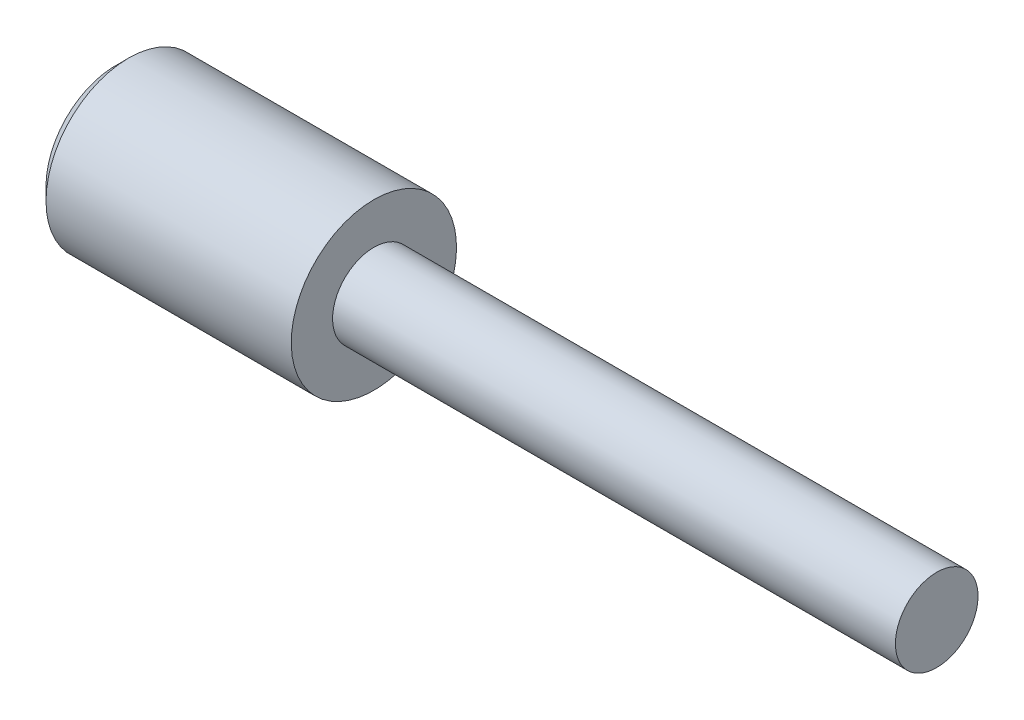
from build123d import *

# Parameters (mm, degrees)
END_CHAMFER_5X45_SIZE = 5


with BuildPart() as part:
    # Shaft Profile → Shaft Body Revolve (revolve)
    with BuildSketch(Plane.XY):
        Polygon((96.878787879, 2.320468839), (-221.121212121, 2.320468839), (-221.121212121, 34.320468839), (-121.121212121, 34.320468839), (-121.121212121, 18.320468839), (96.878787879, 18.320468839), align=None)
    revolve(axis=Axis((96.878787879, 2.320468839, 0), (-1, 0, 0)))

    # End Chamfer 5x45°
    end_chamfer_5x45_edges = [part.edges().sort_by_distance(p)[0] for p in [
        (-221.121212121, -29.679531161, 0),
    ]]
    chamfer(end_chamfer_5x45_edges, length=END_CHAMFER_5X45_SIZE)


solid = part.part
